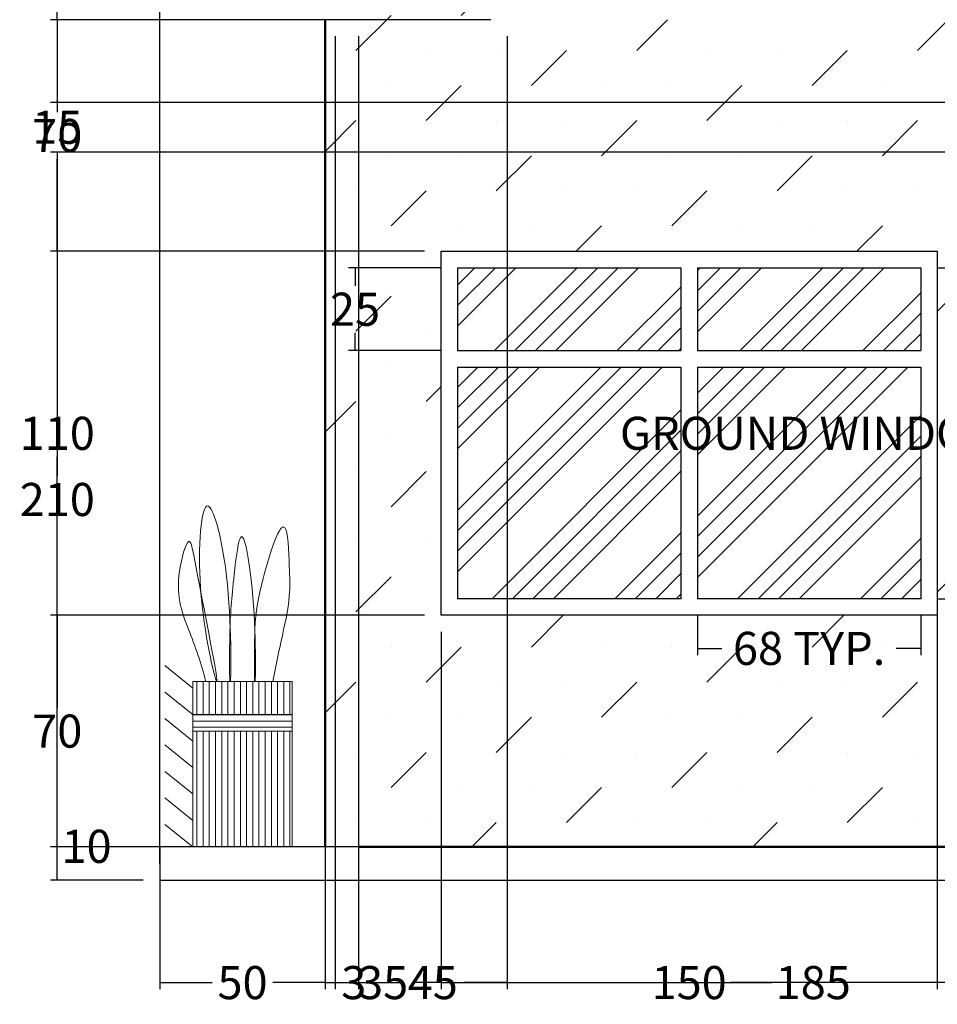
# Model space of a CAD drawing. Units: millimetres. Extents: x 301 to 1039, y -12 to 673.
# Tile 1 of 6: x 301 to 579, y -12 to 285. Entities that reach past the tile are written whole.
import ezdxf

# ---------------------------------------------------------------- set-up
doc = ezdxf.new("R2010")
doc.units = ezdxf.units.MM
doc.header["$MEASUREMENT"] = 0
for name, color, linetype, lineweight in [('A-ANNO-DIMS', 2, 'Continuous', 18), ('A-ELEV', 8, 'Continuous', 25), ('A-GLAZ', 4, 'Continuous', 25), ('A-GLAZ-PATT', 8, 'Continuous', 13), ('A-WALL', 7, 'Continuous', 50), ('A-WALL-PATT', 9, 'Continuous', 13), ('L-PLNT', 3, 'Continuous', 18)]:
    doc.layers.add(name, color=color, linetype=linetype, lineweight=lineweight)
doc.styles.get("Standard").update_dxf_attribs({"font": 'arial.ttf'})
doc.dimstyles.get("Standard").update_dxf_attribs({"dimtxt": 10, "dimasz": 0.18, "dimexe": 2, "dimexo": 5, "dimgap": 2, "dimtad": 0, "dimtih": 1, "dimtoh": 1, "dimdec": 0, "dimzin": 0, "dimdsep": 46, "dimtxsty": 'Standard', "dimcen": 0.09, "dimadec": 0, "dimazin": 0, "dimtfac": 1, "dimtdec": 0, "dimtofl": 0, "dimtmove": 0, "dimatfit": 3, "dimfxl": 1, "dimtolj": 1, "dimtzin": 0, "dimarcsym": 0})

# ---------------------------------------------------------------- blocks, each defined once
blk = doc.blocks.new('*U3')
blk.add_line((0, 0), (6.81, -8.44))
blk = doc.blocks.new('*U4')
at = {"layer": 'L-PLNT', "color": 0, "linetype": 'ByBlock', "lineweight": -2, "transparency": 16777216, "rotation": 90}
for p in [(1079.45, 89.52), (1079.45, 81.52), (1079.45, 73.52), (1079.45, 65.52), (1079.45, 57.52), (1079.45, 49.52), (1079.45, 41.52)]:
    blk.add_blockref('*U3', p, dxfattribs=at)
blk = doc.blocks.new('WIN-SASH-GROUND')
for p, q in [((506.29, 210.09), (506.29, 185.09)), ((506.29, 210.09), (573.79, 210.09)), ((573.79, 210.09), (573.79, 185.09)), ((506.29, 185.09), (573.79, 185.09)), ((506.29, 180.09), (506.29, 110.09)), ((506.29, 180.09), (573.79, 180.09)), ((573.79, 180.09), (573.79, 110.09)), ((573.79, 110.09), (506.29, 110.09))]:
    blk.add_line(p, q)
blk = doc.blocks.new('PLANTER-TALL')
for p, q in [((913.79, 35.09), (913.79, 85.09)), ((913.79, 85.09), (943.79, 85.09)), ((943.79, 85.09), (943.79, 35.09)), ((913.79, 75.09), (943.79, 75.09)), ((913.79, 70.09), (943.79, 70.09))]:
    blk.add_line(p, q)
for points, knots in [([(932.44, 85.09), (932.19, 88.91), (932, 117.56), (940.64, 148.58), (943.41, 110.75), (932.62, 67.84), (940.69, 108.37), (944.93, 130.41), (949.97, 112.97), (945.67, 102.5), (941.16, 90.48), (939.89, 85.09)], [190.612749, 190.612749, 190.612749, 190.612749, 217.894774, 237.177461, 261.995493, 290.738764, 329.494028, 333.833671, 341.635675, 361.055373, 377.63197, 377.63197, 377.63197, 377.63197]), ([(919.6, 85.09), (918.81, 89.12), (917.13, 97.69), (914.28, 109.64), (914.65, 119.96), (915.42, 140.89), (924.57, 111.13), (925.2, 100.17), (925.2, 87.12), (925.13, 85.09)], [0, 0, 0, 0, 12.444322, 26.420596, 35.223716, 47.132736, 67.219262, 83.208341, 95.201321, 95.201321, 95.201321, 95.201321]), ([(924.96, 85.09), (924.77, 89.03), (924.72, 111.77), (929.35, 134.6), (931.92, 112.35), (932.77, 102.84), (932.74, 87.27), (932.64, 85.09)], [102.717678, 102.717678, 102.717678, 102.717678, 128.408935, 139.329582, 151.017137, 169.163832, 183.363914, 183.363914, 183.363914, 183.363914])]:
    blk.add_open_spline(points, degree=3, knots=knots)
blk = doc.blocks.new('*D14')
at = {"layer": 'A-ANNO-DIMS', "color": 0, "lineweight": -2, "transparency": 16777216}
for p, q in [((578.79, 210.09), (590.79, 210.09)), ((588.79, 209.91), (588.79, 167.26)), ((588.79, 110.27), (588.79, 152.91)), ((578.79, 110.09), (590.79, 110.09))]:
    blk.add_line(p, q, dxfattribs=at)
at = {"layer": 'A-ANNO-DIMS', "color": 0, "transparency": 16777216}
for points in [[(588.76, 209.91), (588.82, 209.91), (588.79, 210.09)], [(588.76, 110.27), (588.82, 110.27), (588.79, 110.09)]]:
    blk.add_solid(points, dxfattribs=at)
at = {"layer": 'Defpoints', "color": 0, "transparency": 16777216}
for p in [(573.79, 210.09), (588.79, 210.09), (573.79, 110.09)]:
    blk.add_point(p, dxfattribs=at)
at = {"layer": 'A-ANNO-DIMS', "color": 0, "transparency": 16777216, "insert": (588.79, 160.09), "char_height": 10, "attachment_point": 5}
blk.add_mtext('\\A1;GROUND WINDOW SASH 100 TYP.', dxfattribs=at)
blk = doc.blocks.new('*D15')
at = {"layer": 'A-ANNO-DIMS', "color": 0, "lineweight": -2, "transparency": 16777216}
for p, q in [((506.29, 105.09), (506.29, 93.09)), ((573.79, 105.09), (573.79, 93.09)), ((506.47, 95.09), (513.67, 95.09)), ((573.61, 95.09), (566.4, 95.09))]:
    blk.add_line(p, q, dxfattribs=at)
at = {"layer": 'A-ANNO-DIMS', "color": 0, "transparency": 16777216}
for points in [[(506.47, 95.12), (506.47, 95.06), (506.29, 95.09)], [(573.61, 95.12), (573.61, 95.06), (573.79, 95.09)]]:
    blk.add_solid(points, dxfattribs=at)
at = {"layer": 'Defpoints', "color": 0, "transparency": 16777216}
for p in [(506.29, 110.09), (573.79, 110.09), (573.79, 95.09)]:
    blk.add_point(p, dxfattribs=at)
at = {"layer": 'A-ANNO-DIMS', "color": 0, "transparency": 16777216, "insert": (540.04, 95.09), "char_height": 10, "attachment_point": 5}
blk.add_mtext('\\A1;68 TYP.', dxfattribs=at)
blk = doc.blocks.new('*D20')
at = {"layer": 'A-ANNO-DIMS', "color": 0, "lineweight": -2, "transparency": 16777216}
for p, q in [((343.79, 30.09), (343.79, 668.09)), ((953.79, 30.09), (953.79, 668.09)), ((343.97, 666.09), (635.73, 666.09)), ((953.61, 666.09), (661.85, 666.09))]:
    blk.add_line(p, q, dxfattribs=at)
at = {"layer": 'A-ANNO-DIMS', "color": 0, "transparency": 16777216}
for points in [[(343.97, 666.12), (343.97, 666.06), (343.79, 666.09)], [(953.61, 666.12), (953.61, 666.06), (953.79, 666.09)]]:
    blk.add_solid(points, dxfattribs=at)
at = {"layer": 'Defpoints', "color": 0, "transparency": 16777216}
for p in [(953.79, 666.09), (343.79, 25.09), (953.79, 25.09)]:
    blk.add_point(p, dxfattribs=at)
at = {"layer": 'A-ANNO-DIMS', "color": 0, "transparency": 16777216, "insert": (648.79, 666.09), "char_height": 10, "attachment_point": 5}
blk.add_mtext('\\A1;610', dxfattribs=at)
blk = doc.blocks.new('*D22')
at = {"layer": 'A-ANNO-DIMS', "color": 0, "lineweight": -2, "transparency": 16777216}
for p, q in [((343.79, 30.09), (343.79, -7.91)), ((393.79, 30.09), (393.79, -7.91)), ((343.97, -5.91), (359.64, -5.91)), ((393.61, -5.91), (377.93, -5.91))]:
    blk.add_line(p, q, dxfattribs=at)
at = {"layer": 'A-ANNO-DIMS', "color": 0, "transparency": 16777216}
for points in [[(343.97, -5.88), (343.97, -5.94), (343.79, -5.91)], [(393.61, -5.88), (393.61, -5.94), (393.79, -5.91)]]:
    blk.add_solid(points, dxfattribs=at)
at = {"layer": 'Defpoints', "color": 0, "transparency": 16777216}
for p in [(343.79, 35.09), (393.79, 35.09), (393.79, -5.91)]:
    blk.add_point(p, dxfattribs=at)
at = {"layer": 'A-ANNO-DIMS', "color": 0, "transparency": 16777216, "insert": (368.79, -5.91), "char_height": 10, "attachment_point": 5}
blk.add_mtext('\\A1;50', dxfattribs=at)
blk = doc.blocks.new('*D23')
at = {"layer": 'A-ANNO-DIMS', "color": 0, "lineweight": -2, "transparency": 16777216}
for p, q in [((428.79, 100.09), (428.79, -7.91)), ((393.79, 30.09), (393.79, -7.91)), ((393.97, -5.91), (402.09, -5.91)), ((428.61, -5.91), (420.48, -5.91))]:
    blk.add_line(p, q, dxfattribs=at)
at = {"layer": 'A-ANNO-DIMS', "color": 0, "transparency": 16777216}
for points in [[(393.97, -5.88), (393.97, -5.94), (393.79, -5.91)], [(428.61, -5.88), (428.61, -5.94), (428.79, -5.91)]]:
    blk.add_solid(points, dxfattribs=at)
at = {"layer": 'Defpoints', "color": 0, "transparency": 16777216}
for p in [(428.79, 105.09), (393.79, 35.09), (428.79, -5.91)]:
    blk.add_point(p, dxfattribs=at)
at = {"layer": 'A-ANNO-DIMS', "color": 0, "transparency": 16777216, "insert": (411.29, -5.91), "char_height": 10, "attachment_point": 5}
blk.add_mtext('\\A1;35', dxfattribs=at)
blk = doc.blocks.new('*D24')
at = {"layer": 'A-ANNO-DIMS', "color": 0, "lineweight": -2, "transparency": 16777216}
for p, q in [((578.79, 210.09), (578.79, -7.91)), ((428.79, 100.09), (428.79, -7.91)), ((428.97, -5.91), (491.23, -5.91)), ((578.61, -5.91), (516.35, -5.91))]:
    blk.add_line(p, q, dxfattribs=at)
at = {"layer": 'A-ANNO-DIMS', "color": 0, "transparency": 16777216}
for points in [[(428.97, -5.88), (428.97, -5.94), (428.79, -5.91)], [(578.61, -5.88), (578.61, -5.94), (578.79, -5.91)]]:
    blk.add_solid(points, dxfattribs=at)
at = {"layer": 'Defpoints', "color": 0, "transparency": 16777216}
for p in [(578.79, 215.09), (428.79, 105.09), (578.79, -5.91)]:
    blk.add_point(p, dxfattribs=at)
at = {"layer": 'A-ANNO-DIMS', "color": 0, "transparency": 16777216, "insert": (503.79, -5.91), "char_height": 10, "attachment_point": 5}
blk.add_mtext('\\A1;150', dxfattribs=at)
blk = doc.blocks.new('*D31')
at = {"layer": 'A-ANNO-DIMS', "color": 0, "lineweight": -2, "transparency": 16777216}
for p, q in [((338.79, 35.09), (310.79, 35.09)), ((312.79, 35.09), (312.79, 35.27)), ((312.79, 35.27), (312.97, 35.27)), ((312.79, 25.27), (312.79, 34.91)), ((338.79, 25.09), (310.79, 25.09))]:
    blk.add_line(p, q, dxfattribs=at)
at = {"layer": 'A-ANNO-DIMS', "color": 0, "transparency": 16777216}
for points in [[(312.76, 34.91), (312.82, 34.91), (312.79, 35.09)], [(312.76, 25.27), (312.82, 25.27), (312.79, 25.09)]]:
    blk.add_solid(points, dxfattribs=at)
at = {"layer": 'Defpoints', "color": 0, "transparency": 16777216}
for p in [(312.79, 35.09), (343.79, 35.09), (343.79, 25.09)]:
    blk.add_point(p, dxfattribs=at)
at = {"layer": 'A-ANNO-DIMS', "color": 0, "transparency": 16777216, "insert": (321.64, 35.27), "char_height": 10, "attachment_point": 5}
blk.add_mtext('\\A1;10', dxfattribs=at)
blk = doc.blocks.new('*D32')
at = {"layer": 'A-ANNO-DIMS', "color": 0, "lineweight": -2, "transparency": 16777216}
for p, q in [((423.79, 105.09), (310.79, 105.09)), ((312.79, 104.91), (312.79, 77.19)), ((312.79, 35.27), (312.79, 62.98)), ((388.79, 35.09), (310.79, 35.09))]:
    blk.add_line(p, q, dxfattribs=at)
at = {"layer": 'A-ANNO-DIMS', "color": 0, "transparency": 16777216}
for points in [[(312.76, 104.91), (312.82, 104.91), (312.79, 105.09)], [(312.76, 35.27), (312.82, 35.27), (312.79, 35.09)]]:
    blk.add_solid(points, dxfattribs=at)
at = {"layer": 'Defpoints', "color": 0, "transparency": 16777216}
for p in [(312.79, 105.09), (428.79, 105.09), (393.79, 35.09)]:
    blk.add_point(p, dxfattribs=at)
at = {"layer": 'A-ANNO-DIMS', "color": 0, "transparency": 16777216, "insert": (312.79, 70.09), "char_height": 10, "attachment_point": 5}
blk.add_mtext('\\A1;70', dxfattribs=at)
blk = doc.blocks.new('*D33')
at = {"layer": 'A-ANNO-DIMS', "color": 0, "lineweight": -2, "transparency": 16777216}
for p, q in [((423.79, 215.09), (310.79, 215.09)), ((312.79, 214.91), (312.79, 167.19)), ((312.79, 105.27), (312.79, 152.98)), ((423.79, 105.09), (310.79, 105.09))]:
    blk.add_line(p, q, dxfattribs=at)
at = {"layer": 'A-ANNO-DIMS', "color": 0, "transparency": 16777216}
for points in [[(312.76, 214.91), (312.82, 214.91), (312.79, 215.09)], [(312.76, 105.27), (312.82, 105.27), (312.79, 105.09)]]:
    blk.add_solid(points, dxfattribs=at)
at = {"layer": 'Defpoints', "color": 0, "transparency": 16777216}
for p in [(312.79, 215.09), (428.79, 215.09), (428.79, 105.09)]:
    blk.add_point(p, dxfattribs=at)
at = {"layer": 'A-ANNO-DIMS', "color": 0, "transparency": 16777216, "insert": (312.79, 160.09), "char_height": 10, "attachment_point": 5}
blk.add_mtext('\\A1;110', dxfattribs=at)
blk = doc.blocks.new('*D34')
at = {"layer": 'A-ANNO-DIMS', "color": 0, "lineweight": -2, "transparency": 16777216}
for p, q in [((388.79, 285.09), (310.79, 285.09)), ((312.79, 284.91), (312.79, 257.19)), ((312.79, 215.27), (312.79, 242.98)), ((423.79, 215.09), (310.79, 215.09))]:
    blk.add_line(p, q, dxfattribs=at)
at = {"layer": 'A-ANNO-DIMS', "color": 0, "transparency": 16777216}
for points in [[(312.76, 284.91), (312.82, 284.91), (312.79, 285.09)], [(312.76, 215.27), (312.82, 215.27), (312.79, 215.09)]]:
    blk.add_solid(points, dxfattribs=at)
at = {"layer": 'Defpoints', "color": 0, "transparency": 16777216}
for p in [(312.79, 285.09), (393.79, 285.09), (428.79, 215.09)]:
    blk.add_point(p, dxfattribs=at)
at = {"layer": 'A-ANNO-DIMS', "color": 0, "transparency": 16777216, "insert": (312.79, 250.09), "char_height": 10, "attachment_point": 5}
blk.add_mtext('\\A1;70', dxfattribs=at)
blk = doc.blocks.new('*D35')
at = {"layer": 'A-ANNO-DIMS', "color": 0, "lineweight": -2, "transparency": 16777216}
for p, q in [((388.79, 505.09), (310.79, 505.09)), ((312.79, 504.91), (312.79, 402.19)), ((312.79, 285.27), (312.79, 387.98)), ((388.79, 285.09), (310.79, 285.09))]:
    blk.add_line(p, q, dxfattribs=at)
at = {"layer": 'A-ANNO-DIMS', "color": 0, "transparency": 16777216}
for points in [[(312.76, 504.91), (312.82, 504.91), (312.79, 505.09)], [(312.76, 285.27), (312.82, 285.27), (312.79, 285.09)]]:
    blk.add_solid(points, dxfattribs=at)
at = {"layer": 'Defpoints', "color": 0, "transparency": 16777216}
for p in [(312.79, 505.09), (393.79, 505.09), (393.79, 285.09)]:
    blk.add_point(p, dxfattribs=at)
at = {"layer": 'A-ANNO-DIMS', "color": 0, "transparency": 16777216, "insert": (312.79, 395.09), "char_height": 10, "attachment_point": 5}
blk.add_mtext('\\A1;220', dxfattribs=at)
blk = doc.blocks.new('*D37')
at = {"layer": 'A-ANNO-DIMS', "color": 0, "lineweight": -2, "transparency": 16777216}
for p, q in [((428.79, 210.09), (400.79, 210.09)), ((402.79, 209.91), (402.79, 204.69)), ((402.79, 185.27), (402.79, 190.48)), ((428.79, 185.09), (400.79, 185.09))]:
    blk.add_line(p, q, dxfattribs=at)
at = {"layer": 'A-ANNO-DIMS', "color": 0, "transparency": 16777216}
for points in [[(402.76, 209.91), (402.82, 209.91), (402.79, 210.09)], [(402.76, 185.27), (402.82, 185.27), (402.79, 185.09)]]:
    blk.add_solid(points, dxfattribs=at)
at = {"layer": 'Defpoints', "color": 0, "transparency": 16777216}
for p in [(402.79, 210.09), (433.79, 210.09), (433.79, 185.09)]:
    blk.add_point(p, dxfattribs=at)
at = {"layer": 'A-ANNO-DIMS', "color": 0, "transparency": 16777216, "insert": (402.79, 197.59), "char_height": 10, "attachment_point": 5}
blk.add_mtext('\\A1;25', dxfattribs=at)
blk = doc.blocks.new('*D50')
at = {"layer": 'A-ANNO-DIMS', "color": 0, "lineweight": -2, "transparency": 16777216}
for p, q in [((403.79, 280.09), (403.79, -7.91)), ((448.79, 280.09), (448.79, -7.91)), ((403.97, -5.91), (416.89, -5.91)), ((448.61, -5.91), (435.69, -5.91))]:
    blk.add_line(p, q, dxfattribs=at)
at = {"layer": 'A-ANNO-DIMS', "color": 0, "transparency": 16777216}
for points in [[(403.97, -5.88), (403.97, -5.94), (403.79, -5.91)], [(448.61, -5.88), (448.61, -5.94), (448.79, -5.91)]]:
    blk.add_solid(points, dxfattribs=at)
at = {"layer": 'Defpoints', "color": 0, "transparency": 16777216}
for p in [(403.79, 285.09), (448.79, 285.09), (448.79, -5.91)]:
    blk.add_point(p, dxfattribs=at)
at = {"layer": 'A-ANNO-DIMS', "color": 0, "transparency": 16777216, "insert": (426.29, -5.91), "char_height": 10, "attachment_point": 5}
blk.add_mtext('\\A1;45', dxfattribs=at)
blk = doc.blocks.new('*D51')
at = {"layer": 'A-ANNO-DIMS', "color": 0, "lineweight": -2, "transparency": 16777216}
for p, q in [((448.79, 280.09), (448.79, -7.91)), ((633.79, 280.09), (633.79, -7.91)), ((448.97, -5.91), (528.67, -5.91)), ((633.61, -5.91), (553.9, -5.91))]:
    blk.add_line(p, q, dxfattribs=at)
at = {"layer": 'A-ANNO-DIMS', "color": 0, "transparency": 16777216}
for points in [[(448.97, -5.88), (448.97, -5.94), (448.79, -5.91)], [(633.61, -5.88), (633.61, -5.94), (633.79, -5.91)]]:
    blk.add_solid(points, dxfattribs=at)
at = {"layer": 'Defpoints', "color": 0, "transparency": 16777216}
for p in [(448.79, 285.09), (633.79, 285.09), (633.79, -5.91)]:
    blk.add_point(p, dxfattribs=at)
at = {"layer": 'A-ANNO-DIMS', "color": 0, "transparency": 16777216, "insert": (541.29, -5.91), "char_height": 10, "attachment_point": 5}
blk.add_mtext('\\A1;185', dxfattribs=at)
blk = doc.blocks.new('*D54')
at = {"layer": 'A-ANNO-DIMS', "color": 0, "lineweight": -2, "transparency": 16777216}
for p, q in [((393.79, 280.09), (393.79, -7.91)), ((396.79, 280.09), (396.79, -7.91)), ((393.61, -5.91), (393.43, -5.91)), ((396.97, -5.91), (397.15, -5.91))]:
    blk.add_line(p, q, dxfattribs=at)
at = {"layer": 'A-ANNO-DIMS', "color": 0, "transparency": 16777216}
for points in [[(393.61, -5.88), (393.61, -5.94), (393.79, -5.91)], [(396.97, -5.88), (396.97, -5.94), (396.79, -5.91)]]:
    blk.add_solid(points, dxfattribs=at)
at = {"layer": 'Defpoints', "color": 0, "transparency": 16777216}
for p in [(393.79, 285.09), (396.79, 285.09), (396.79, -5.91)]:
    blk.add_point(p, dxfattribs=at)
at = {"layer": 'A-ANNO-DIMS', "color": 0, "transparency": 16777216, "insert": (402.42, -5.91), "char_height": 10, "attachment_point": 5}
blk.add_mtext('\\A1;3', dxfattribs=at)
blk = doc.blocks.new('*D58')
at = {"layer": 'A-ANNO-DIMS', "color": 0, "lineweight": -2, "transparency": 16777216}
for p, q in [((443.79, 440.09), (310.79, 440.09)), ((312.79, 439.91), (312.79, 369.69)), ((312.79, 285.27), (312.79, 355.48)), ((443.79, 285.09), (310.79, 285.09))]:
    blk.add_line(p, q, dxfattribs=at)
at = {"layer": 'A-ANNO-DIMS', "color": 0, "transparency": 16777216}
for points in [[(312.76, 439.91), (312.82, 439.91), (312.79, 440.09)], [(312.76, 285.27), (312.82, 285.27), (312.79, 285.09)]]:
    blk.add_solid(points, dxfattribs=at)
at = {"layer": 'Defpoints', "color": 0, "transparency": 16777216}
for p in [(312.79, 440.09), (448.79, 440.09), (448.79, 285.09)]:
    blk.add_point(p, dxfattribs=at)
at = {"layer": 'A-ANNO-DIMS', "color": 0, "transparency": 16777216, "insert": (312.79, 362.59), "char_height": 10, "attachment_point": 5}
blk.add_mtext('\\A1;155', dxfattribs=at)
blk = doc.blocks.new('*D64')
at = {"layer": 'A-ANNO-DIMS', "color": 0, "lineweight": -2, "transparency": 16777216}
for p, q in [((608.79, 245.09), (310.79, 245.09)), ((312.79, 244.91), (312.79, 147.19)), ((312.79, 35.27), (312.79, 132.98)), ((608.79, 35.09), (310.79, 35.09))]:
    blk.add_line(p, q, dxfattribs=at)
at = {"layer": 'A-ANNO-DIMS', "color": 0, "transparency": 16777216}
for points in [[(312.76, 244.91), (312.82, 244.91), (312.79, 245.09)], [(312.76, 35.27), (312.82, 35.27), (312.79, 35.09)]]:
    blk.add_solid(points, dxfattribs=at)
at = {"layer": 'Defpoints', "color": 0, "transparency": 16777216}
for p in [(312.79, 245.09), (613.79, 245.09), (613.79, 35.09)]:
    blk.add_point(p, dxfattribs=at)
at = {"layer": 'A-ANNO-DIMS', "color": 0, "transparency": 16777216, "insert": (312.79, 140.09), "char_height": 10, "attachment_point": 5}
blk.add_mtext('\\A1;210', dxfattribs=at)
blk = doc.blocks.new('*D65')
at = {"layer": 'A-ANNO-DIMS', "color": 0, "lineweight": -2, "transparency": 16777216}
for p, q in [((608.788413, 260.088152), (310.788413, 260.088152)), ((312.788413, 260.268152), (312.788413, 260.448152)), ((608.788413, 245.088152), (310.788413, 245.088152)), ((312.788413, 244.908152), (312.788413, 244.728152))]:
    blk.add_line(p, q, dxfattribs=at)
at = {"layer": 'A-ANNO-DIMS', "color": 0, "transparency": 16777216}
for points in [[(312.758413, 260.268152), (312.818413, 260.268152), (312.788413, 260.088152)], [(312.758413, 244.908152), (312.818413, 244.908152), (312.788413, 245.088152)]]:
    blk.add_solid(points, dxfattribs=at)
at = {"layer": 'Defpoints', "color": 0, "transparency": 16777216}
for p in [(312.788413, 260.088152), (613.788413, 260.088152), (613.788413, 245.088152)]:
    blk.add_point(p, dxfattribs=at)
at = {"layer": 'A-ANNO-DIMS', "color": 0, "transparency": 16777216, "insert": (312.788413, 252.588152), "char_height": 10, "attachment_point": 5}
blk.add_mtext('\\A1;15', dxfattribs=at)

msp = doc.modelspace()

# ---------------------------------------------------------------- hatches: boundary and pattern name
at = {"layer": 'A-GLAZ-PATT'}
h = msp.add_hatch(dxfattribs=at)
h.set_pattern_fill('ANSI34', color=256, scale=35)
h.paths.add_polyline_path([(528.788, 400.52), (528.788, 425.088), (463.788, 425.088), (463.788, 400.52), (463.788, 335.088), (528.788, 335.088)])
h.paths.add_polyline_path([(494.288, 333.088), (463.788, 333.088), (463.788, 300.088), (494.288, 300.088)])
h.paths.add_polyline_path([(528.788, 333.088), (496.288, 333.088), (496.288, 300.088), (528.788, 300.088)])
h.paths.add_polyline_path([(618.788, 400.52), (618.788, 425.088), (553.788, 425.088), (553.788, 400.52), (553.788, 335.088), (618.788, 335.088)])
h.paths.add_polyline_path([(618.788, 333.088), (574.798, 333.088), (574.798, 300.088), (618.788, 300.088)])
h.paths.add_polyline_path([(572.798, 333.088), (553.788, 333.088), (553.788, 300.088), (572.798, 300.088)])
h.paths.add_polyline_path([(501.288, 180.088), (433.788, 180.088), (433.788, 110.088), (501.288, 110.088)])
h.paths.add_polyline_path([(573.788, 180.088), (506.288, 180.088), (506.288, 110.088), (573.788, 110.088)])
h.paths.add_polyline_path([(573.788, 210.088), (506.288, 210.088), (506.288, 185.088), (573.788, 185.088)])
h.paths.add_polyline_path([(501.288, 210.088), (433.788, 210.088), (433.788, 185.088), (501.288, 185.088)])
h.paths.add_polyline_path([(797.687, 412.264), (746.687, 412.264), (746.687, 298.264), (797.687, 298.264)])
h.paths.add_polyline_path([(860.687, 412.264), (809.687, 412.264), (809.687, 298.264), (860.687, 298.264)])
at = {"layer": 'A-WALL-PATT'}
h = msp.add_hatch(dxfattribs=at)
h.set_pattern_fill('MUDST', color=256, scale=60, angle=45)
edge = h.paths.add_edge_path()
edge.add_line((703.788, 505.088), (403.788, 505.088))
edge.add_line((403.788, 505.088), (403.788, 335.088))
edge.add_line((403.788, 335.088), (448.788, 335.088))
edge.add_line((448.788, 335.088), (448.788, 400.52))
edge.add_line((448.788, 400.52), (448.788, 440.088))
edge.add_line((448.788, 440.088), (633.788, 440.088))
edge.add_line((633.788, 440.088), (633.788, 400.52))
edge.add_line((633.788, 400.52), (633.788, 335.088))
edge.add_line((633.788, 335.088), (673.88, 335.088))
edge.add_spline(control_points=[(673.88, 335.088), (673.929, 335.734), (674.283, 339.462), (675.587, 346.794), (678.602, 339.909), (679.226, 336.718), (679.369, 335.088)], knot_values=[26.7052686, 26.7052686, 26.7052686, 26.7052686, 28.3156814, 35.5227919, 39.6456178, 44.5318346, 44.5318346, 44.5318346, 44.5318346], degree=3, periodic=0)
edge.add_line((679.369, 335.088), (703.788, 335.088))
edge.add_line((703.788, 335.088), (703.788, 505.088))
h.paths.add_polyline_path([(681.292, 397.334, -1), (651.292, 397.334, -1)], flags=16)
h.paths.add_polyline_path([(679.292, 397.334, -1), (653.292, 397.334, -1)], flags=0)
h.paths.add_polyline_path([(448.788, 333.088), (403.788, 333.088), (403.788, 285.088), (448.788, 285.088)])
h.paths.add_polyline_path([(613.788, 260.088), (713.788, 260.088), (713.788, 285.088), (403.788, 285.088), (393.788, 285.088), (393.788, 35.088), (403.788, 35.088), (613.788, 35.088)])
h.paths.add_polyline_path([(578.788, 215.088), (578.788, 105.088), (428.788, 105.088), (428.788, 215.088)], flags=16)
h.paths.add_polyline_path([(501.288, 210.088), (501.288, 185.088), (433.788, 185.088), (433.788, 210.088)], flags=0)
h.paths.add_polyline_path([(501.288, 180.088), (501.288, 110.088), (433.788, 110.088), (433.788, 180.088)], flags=0)
h.paths.add_polyline_path([(506.288, 210.088), (573.788, 210.088), (573.788, 185.088), (506.288, 185.088)], flags=0)
h.paths.add_polyline_path([(506.288, 180.088), (573.788, 180.088), (573.788, 110.088), (506.288, 110.088)], flags=0)
edge = h.paths.add_edge_path()
edge.add_spline(control_points=[(675.148, 309.006), (675.282, 309.92), (671.965, 311.304), (670.019, 313.17), (668.379, 316.485), (667.076, 320.028), (669.149, 324.142), (672.687, 322.877), (673.644, 321.553), (673.786, 321.296)], knot_values=[12.4980994, 12.4980994, 12.4980994, 12.4980994, 15.7345293, 18.1242776, 22.0598536, 26.1694355, 29.2709867, 33.3603853, 34.273637, 34.273637, 34.273637, 34.273637], degree=3, periodic=0)
edge.add_spline(control_points=[(673.786, 321.296), (673.373, 322.666), (672.565, 324.662), (673.805, 325.84), (674.246, 326.099)], knot_values=[12.3304253, 12.3304253, 12.3304253, 12.3304253, 16.1943692, 17.6683934, 17.6683934, 17.6683934, 17.6683934], degree=3, periodic=0)
edge.add_spline(control_points=[(674.246, 326.099), (673.92, 328.298), (673.697, 330.39), (673.774, 333.088)], knot_values=[46.2924512, 46.2924512, 46.2924512, 46.2924512, 53.8278009, 53.8278009, 53.8278009, 53.8278009], degree=3, periodic=0)
edge.add_line((673.774, 333.088), (648.788, 333.088))
edge.add_line((648.788, 333.088), (648.788, 285.088))
edge.add_line((648.788, 285.088), (666.788, 285.088))
edge.add_line((666.788, 285.088), (664.215, 309.96))
edge.add_arc((676.288, 385.148), 76.15, 260.87778, 269.14183)
edge = h.paths.add_edge_path()
edge.add_line((703.788, 333.088), (679.453, 333.088))
edge.add_spline(control_points=[(679.453, 333.088), (679.452, 331.277), (679.21, 329.205), (678.936, 327.067), (678.889, 326.706)], knot_values=[17.8386285, 17.8386285, 17.8386285, 17.8386285, 23.5111371, 24.6594022, 24.6594022, 24.6594022, 24.6594022], degree=3, periodic=0)
edge.add_spline(control_points=[(678.889, 326.706), (678.729, 326.741), (678.565, 326.771), (678.396, 326.794)], knot_values=[21.2892091, 21.2892091, 21.2892091, 21.2892091, 21.7264211, 21.7264211, 21.7264211, 21.7264211], degree=3, periodic=0)
edge.add_spline(control_points=[(678.396, 326.794), (678.233, 326.816), (678.067, 326.832), (677.898, 326.842)], knot_values=[20.8675669, 20.8675669, 20.8675669, 20.8675669, 21.2892091, 21.2892091, 21.2892091, 21.2892091], degree=3, periodic=0)
edge.add_spline(control_points=[(677.898, 326.842), (676.995, 326.898), (676.024, 326.786), (675.195, 326.517)], knot_values=[18.611077, 18.611077, 18.611077, 18.611077, 20.8675669, 20.8675669, 20.8675669, 20.8675669], degree=3, periodic=0)
edge.add_spline(control_points=[(675.195, 326.517), (675.029, 326.464), (674.869, 326.404), (674.716, 326.337)], knot_values=[18.1593829, 18.1593829, 18.1593829, 18.1593829, 18.611077, 18.611077, 18.611077, 18.611077], degree=3, periodic=0)
edge.add_spline(control_points=[(674.716, 326.337), (674.55, 326.265), (674.392, 326.186), (674.246, 326.099)], knot_values=[17.6683934, 17.6683934, 17.6683934, 17.6683934, 18.1593829, 18.1593829, 18.1593829, 18.1593829], degree=3, periodic=0)
edge.add_spline(control_points=[(674.246, 326.099), (673.805, 325.84), (672.565, 324.662), (673.373, 322.666), (673.786, 321.296)], knot_values=[12.3304253, 12.3304253, 12.3304253, 12.3304253, 13.8044495, 17.6683934, 17.6683934, 17.6683934, 17.6683934], degree=3, periodic=0)
edge.add_spline(control_points=[(673.786, 321.296), (674.162, 320.613), (674.301, 319.823), (674.341, 318.987)], knot_values=[10.0649388, 10.0649388, 10.0649388, 10.0649388, 12.4980994, 12.4980994, 12.4980994, 12.4980994], degree=3, periodic=0)
edge.add_spline(control_points=[(674.341, 318.987), (674.206, 319.737), (674.024, 320.504), (673.786, 321.296)], knot_values=[10.094462, 10.094462, 10.094462, 10.094462, 12.3304253, 12.3304253, 12.3304253, 12.3304253], degree=3, periodic=0)
edge.add_spline(control_points=[(673.786, 321.296), (673.644, 321.553), (672.687, 322.877), (669.149, 324.142), (667.076, 320.028), (668.379, 316.485), (670.019, 313.17), (671.965, 311.304), (675.282, 309.92), (675.148, 309.006)], knot_values=[12.4980994, 12.4980994, 12.4980994, 12.4980994, 13.4113511, 17.5007497, 20.6023009, 24.7118828, 28.6474588, 31.0372071, 34.273637, 34.273637, 34.273637, 34.273637], degree=3, periodic=0)
edge.add_arc((676.288, 385.148), 76.15, 260.87778, 269.14183, ccw=False)
edge.add_line((664.215, 309.96), (666.788, 285.088))
edge.add_line((666.788, 285.088), (703.788, 285.088))
edge.add_line((703.788, 285.088), (703.788, 333.088))
h.paths.add_polyline_path([(687.234, 308.777), (684.887, 286.088), (667.69, 286.088), (665.343, 308.777, 0.0712952)], flags=16)
h.paths.add_polyline_path([(903.788, 265.672), (713.788, 265.672), (713.788, 260.088), (703.788, 260.088), (703.788, 35.088), (728.788, 35.088), (728.788, 160.088), (878.788, 160.088), (878.788, 35.088), (903.788, 35.088)])
at = {"layer": 'L-PLNT'}
h = msp.add_hatch(dxfattribs=at)
h.set_pattern_fill('ANSI31', color=256, scale=15, angle=45)
h.set_pattern_definition([(90, (-560, 0), (-1.875, 0), [])])
edge = h.paths.add_edge_path()
edge.add_line((383.788, 85.088), (376.592, 85.088))
edge.add_spline(control_points=[(376.592, 85.088), (376.558, 85.041), (376.535, 85.042), (376.521, 85.088)], knot_values=[290.7387637, 290.7387637, 290.7387637, 290.7387637, 292.5163462, 292.5163462, 292.5163462, 292.5163462], degree=3, periodic=0)
edge.add_line((376.521, 85.088), (353.788, 85.088))
edge.add_line((353.788, 85.088), (353.788, 75.088))
edge.add_line((353.788, 75.088), (383.788, 75.088))
edge.add_line((383.788, 75.088), (383.788, 85.088))
h.paths.add_polyline_path([(383.788, 70.088), (353.788, 70.088), (353.788, 35.088), (383.788, 35.088)])
h = msp.add_hatch(dxfattribs=at)
h.set_pattern_fill('ANSI31', color=256, scale=15, angle=135)
h.set_pattern_definition([(180, (-560, 0), (-1e-16, -1.875), [])])
h.paths.add_polyline_path([(383.788, 75.088), (353.788, 75.088), (353.788, 70.088), (383.788, 70.088)])

# ---------------------------------------------------------------- linework, layer by layer
at = {"layer": 'A-ELEV'}
for p, q in [((403.788, 35.088), (343.788, 35.088)), ((343.788, 35.088), (343.788, 25.088)), ((343.788, 25.088), (403.788, 25.088)), ((403.788, 25.088), (618.788, 25.088))]:
    msp.add_line(p, q, dxfattribs=at)
at = {"layer": 'A-GLAZ'}
for p, q in [((428.788, 215.088), (578.788, 215.088)), ((428.788, 105.088), (428.788, 215.088)), ((578.788, 215.088), (578.788, 105.088)), ((578.788, 105.088), (428.788, 105.088))]:
    msp.add_line(p, q, dxfattribs=at)
at = {"layer": 'A-WALL'}
for p, q in [((393.788, 285.088), (393.788, 35.088)), ((953.788, 35.088), (403.788, 35.088))]:
    msp.add_line(p, q, dxfattribs=at)

# ---------------------------------------------------------------- block references
at = {"layer": 'A-GLAZ'}
for p in [(-72.5, 0), (0, 0)]:
    msp.add_blockref('WIN-SASH-GROUND', p, dxfattribs=at)
at = {"layer": 'L-PLNT', "extrusion": (0, 0, -1), "zscale": -1}
msp.add_blockref('PLANTER-TALL', (-1297.577, 0), dxfattribs=at)
at = {"layer": 'L-PLNT', "xscale": -1}
msp.add_blockref('*U4', (1433.239, -6.433), dxfattribs=at)

# ---------------------------------------------------------------- dimensions: what is measured, and where the dimension line sits
at = {"layer": 'A-ANNO-DIMS'}
for base, p1, p2, picture, middle in [((953.788, 666.088), (343.788, 25.088), (953.788, 25.088), '*D20', (648.788, 666.088)), ((396.788, -5.912), (393.788, 285.088), (396.788, 285.088), '*D54', (402.423, -5.912)), ((448.788, -5.912), (403.788, 285.088), (448.788, 285.088), '*D50', (426.288, -5.912)), ((633.788, -5.912), (448.788, 285.088), (633.788, 285.088), '*D51', (541.288, -5.912)), ((578.788, -5.912), (428.788, 105.088), (578.788, 215.088), '*D24', (503.788, -5.912)), ((428.788, -5.912), (393.788, 35.088), (428.788, 105.088), '*D23', (411.288, -5.912)), ((393.788, -5.912), (343.788, 35.088), (393.788, 35.088), '*D22', (368.788, -5.912))]:
    dim = msp.add_linear_dim(base=base, p1=p1, p2=p2, dimstyle='Standard', override={"dimdec": 0, "dimlfac": 1, "dimrnd": 0, "dimzin": 0, "dimdsep": 46, "dimlunit": 2}, dxfattribs=at)
    dim.commit()
    dim.dimension.update_dxf_attribs({"geometry": picture, "text_midpoint": middle})
for base, p1, p2, picture, middle in [((312.788, 505.088), (393.788, 285.088), (393.788, 505.088), '*D35', (312.788, 395.088)), ((312.788, 440.088), (448.788, 285.088), (448.788, 440.088), '*D58', (312.788, 362.588)), ((312.788, 285.088), (428.788, 215.088), (393.788, 285.088), '*D34', (312.788, 250.088)), ((312.788, 260.088), (613.788, 245.088), (613.788, 260.088), '*D65', (312.788, 252.588)), ((312.788, 245.088), (613.788, 35.088), (613.788, 245.088), '*D64', (312.788, 140.088)), ((312.788, 215.088), (428.788, 105.088), (428.788, 215.088), '*D33', (312.788, 160.088)), ((402.788, 210.088), (433.788, 185.088), (433.788, 210.088), '*D37', (402.788, 197.588)), ((312.788, 105.088), (393.788, 35.088), (428.788, 105.088), '*D32', (312.788, 70.088)), ((312.788, 35.088), (343.788, 25.088), (343.788, 35.088), '*D31', (321.643, 35.268))]:
    dim = msp.add_linear_dim(base=base, p1=p1, p2=p2, angle=90, dimstyle='Standard', override={"dimdec": 0, "dimlfac": 1, "dimrnd": 0, "dimzin": 0, "dimdsep": 46, "dimlunit": 2}, dxfattribs=at)
    dim.commit()
    dim.dimension.update_dxf_attribs({"geometry": picture, "text_midpoint": middle})
dim = msp.add_linear_dim(base=(588.788, 210.088), p1=(573.788, 110.088), p2=(573.788, 210.088), angle=90, text='GROUND WINDOW SASH <> TYP.', dimstyle='Standard', override={"dimdec": 0, "dimrnd": 0, "dimzin": 0, "dimlunit": 2}, dxfattribs=at)
dim.commit()
dim.dimension.update_dxf_attribs({"geometry": '*D14', "text_midpoint": (588.788, 160.088)})
dim = msp.add_linear_dim(base=(573.78841292, 95.088152284), p1=(506.28841292, 110.088152284), p2=(573.78841292, 110.088152284), text='<> TYP.', dimstyle='Standard', override={"dimdec": 0, "dimrnd": 0, "dimzin": 0, "dimlunit": 2}, dxfattribs=at)
dim.commit()
dim.dimension.update_dxf_attribs({"geometry": '*D15', "text_midpoint": (540.03841292, 95.088152284)})

doc.saveas('drawing.dxf')
